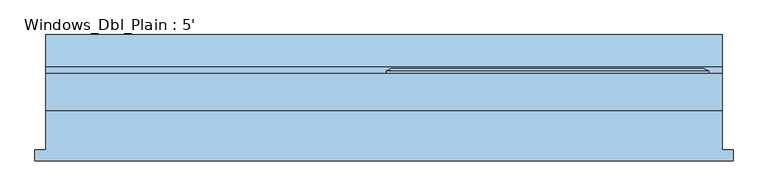
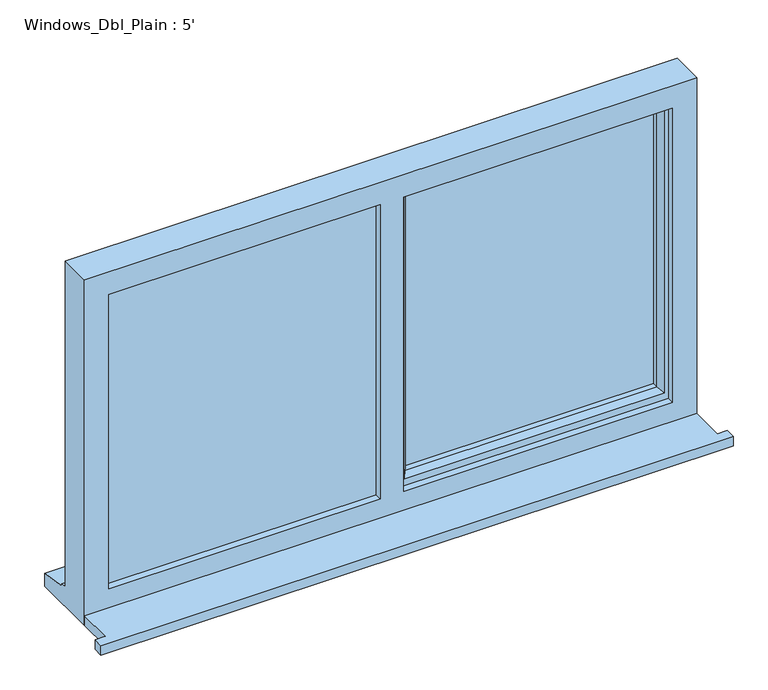
"""IFC4 building model written with IfcOpenShell, lengths in millimetres: window geometry, Windows_Dbl_Plain : 5'."""

from ifc_helpers import new_model, si_unit, frame, origin, place, context, project, spatial, polyline, outline, extrude, faceted_brep, source, transform, mapped, element, save


def windows_dbl_plain_5_93ba300c(model_context):
    return source(origin(), model_context, "Body", "SolidModel", [
        extrude(outline(polyline([(-1072.0, -127.7954322), (-1072.0, -102.7954322), (-1047.0, -102.7954322), (-1047.0, -13.2914322), (477.0, -13.2914322), (477.0, -102.7954322), (502.0, -102.7954322), (502.0, -127.7954322), (-1072.0, -127.7954322)])), frame((0.0, 0.0, 1200.0), z_axis=(0.0, 0.0, 1.0), x_axis=(1.0, 0.0, 0.0)), (0.0, 0.0, 1.0), 25.0),
        faceted_brep([(-280.0, 69.7085678, 2080.0), (-280.0, 75.4820705, 2080.0), (-280.0, 75.4820705, 1253.0), (-280.0, 69.7085678, 1253.0), (-270.0, 4.7085678, 2070.0), (-270.0, 69.7085678, 2070.0), (-270.0, 69.7085678, 1263.0), (-270.0, 4.7085678, 1263.0), (-230.0, 19.2014677, 2030.0), (-240.1480377, 4.7085678, 2040.1480377), (-240.1480377, 4.7085678, 1292.8519623), (-230.0, 19.2014677, 1303.0), (-230.0, 33.7085678, 2030.0), (-230.0, 33.7085678, 1303.0), (-240.0, 57.7085678, 2040.0), (-240.0, 33.7085678, 2040.0), (-240.0, 33.7085678, 1293.0), (-240.0, 57.7085678, 1293.0), (-230.0, 75.4820705, 2030.0), (-230.0, 57.7085678, 2030.0), (-230.0, 57.7085678, 1303.0), (-230.0, 75.4820705, 1303.0), (-247.4457548, 81.2555732, 2047.4457548), (-247.4457548, 81.2555732, 1285.5542452), (-269.2153903, 81.2555732, 2069.2153903), (-269.2153903, 81.2555732, 1263.7846097), (447.0, 75.4820705, 1253.0), (447.0, 69.7085678, 1253.0), (437.0, 69.7085678, 1263.0), (437.0, 4.7085678, 1263.0), (407.1480377, 4.7085678, 1292.8519623), (397.0, 19.2014677, 1303.0), (397.0, 33.7085678, 1303.0), (407.0, 33.7085678, 1293.0), (407.0, 57.7085678, 1293.0), (397.0, 57.7085678, 1303.0), (397.0, 75.4820705, 1303.0), (414.4457548, 81.2555732, 1285.5542452), (436.2153903, 81.2555732, 1263.7846097), (447.0, 75.4820705, 2080.0), (447.0, 69.7085678, 2080.0), (437.0, 69.7085678, 2070.0), (437.0, 4.7085678, 2070.0), (407.1480377, 4.7085678, 2040.1480377), (397.0, 19.2014677, 2030.0), (397.0, 33.7085678, 2030.0), (407.0, 33.7085678, 2040.0), (407.0, 57.7085678, 2040.0), (397.0, 57.7085678, 2030.0), (397.0, 75.4820705, 2030.0), (414.4457548, 81.2555732, 2047.4457548), (436.2153903, 81.2555732, 2069.2153903)], [[[0, 1, 2, 3]], [[4, 5, 6, 7]], [[8, 9, 10, 11]], [[12, 8, 11, 13]], [[14, 15, 16, 17]], [[18, 19, 20, 21]], [[22, 18, 21, 23]], [[1, 24, 25, 2]], [[3, 2, 26, 27]], [[7, 6, 28, 29]], [[11, 10, 30, 31]], [[13, 11, 31, 32]], [[17, 16, 33, 34]], [[21, 20, 35, 36]], [[23, 21, 36, 37]], [[2, 25, 38, 26]], [[27, 26, 39, 40]], [[29, 28, 41, 42]], [[31, 30, 43, 44]], [[32, 31, 44, 45]], [[34, 33, 46, 47]], [[36, 35, 48, 49]], [[37, 36, 49, 50]], [[26, 38, 51, 39]], [[40, 39, 1, 0]], [[3, 27, 40, 0], [5, 41, 28, 6]], [[42, 41, 5, 4]], [[7, 29, 42, 4], [9, 43, 30, 10]], [[44, 43, 9, 8]], [[45, 44, 8, 12]], [[15, 46, 33, 16], [13, 32, 45, 12]], [[47, 46, 15, 14]], [[17, 34, 47, 14], [19, 48, 35, 20]], [[49, 48, 19, 18]], [[50, 49, 18, 22]], [[24, 51, 38, 25], [23, 37, 50, 22]], [[39, 51, 24, 1]]]),
        extrude(outline(polyline([(2050.0, -310.0), (2070.0, -310.0), (2070.0, -1007.0), (1263.0, -1007.0), (1263.0, -310.0), (1283.0, -310.0), (1283.0, -987.0), (2050.0, -987.0), (2050.0, -310.0)])), frame((0.0, 28.7085678, 0.0), z_axis=(0.0, 1.0, 0.0), x_axis=(0.0, 0.0, 1.0)), (0.0, 0.0, 1.0), 41.0),
        faceted_brep([(477.0, -13.2914322, 2110.0), (-1047.0, -13.2914322, 2110.0), (-1047.0, -13.2914322, 1200.0), (477.0, -13.2914322, 1200.0), (417.0, -13.2914322, 2050.0), (417.0, -13.2914322, 1275.0), (-252.0, -13.2914322, 1275.0), (-252.0, -13.2914322, 2050.0), (-310.0, -13.2914322, 2050.0), (-310.0, -13.2914322, 1275.0), (-987.0, -13.2914322, 1275.0), (-987.0, -13.2914322, 2050.0), (-1047.0, 69.7085678, 2110.0), (-1047.0, 69.7085678, 1251.0), (-1047.0, 84.7085678, 1249.68767), (-1047.0, 84.7085678, 1244.7449676), (-1047.0, 157.2085678, 1233.8088847), (-1047.0, 157.2085678, 1200.0), (477.0, 69.7085678, 2110.0), (477.0, 69.7085678, 1251.0), (-1007.0, 69.7085678, 2070.0), (-1007.0, 69.7085678, 1263.0), (-310.0, 69.7085678, 1263.0), (-310.0, 69.7085678, 2070.0), (-270.0, 69.7085678, 2070.0), (-270.0, 69.7085678, 1263.0), (437.0, 69.7085678, 1263.0), (437.0, 69.7085678, 2070.0), (-1007.0, 4.7085678, 2070.0), (-1007.0, 4.7085678, 1263.0), (-300.0, 4.7085678, 2070.0), (-300.0, 4.7085678, 1263.0), (-310.0, 4.7085678, 2050.0), (-987.0, 4.7085678, 2050.0), (-987.0, 4.7085678, 1275.0), (-310.0, 4.7085678, 1275.0), (-270.0, 4.7085678, 2070.0), (437.0, 4.7085678, 2070.0), (437.0, 4.7085678, 1263.0), (-270.0, 4.7085678, 1263.0), (417.0, 4.7085678, 2050.0), (-252.0, 4.7085678, 2050.0), (-252.0, 4.7085678, 1275.0), (417.0, 4.7085678, 1275.0), (-310.0, 28.7085678, 2070.0), (-300.0, 28.7085678, 2070.0), (477.0, 157.2085678, 1200.0), (477.0, 157.2085678, 1233.8088847), (477.0, 84.7085678, 1244.7449676), (477.0, 84.7085678, 1249.68767), (-300.0, 28.7085678, 1263.0), (-310.0, 28.7085678, 1263.0)], [[[0, 1, 2, 3], [4, 5, 6, 7], [8, 9, 10, 11]], [[2, 1, 12, 13, 14, 15, 16, 17]], [[13, 12, 18, 19], [20, 21, 22, 23], [24, 25, 26, 27]], [[21, 20, 28, 29]], [[28, 30, 31, 29], [32, 33, 34, 35]], [[36, 37, 38, 39], [40, 41, 42, 43]], [[33, 11, 10, 34]], [[1, 0, 18, 12]], [[28, 20, 23, 44, 45, 30]], [[27, 37, 36, 24]], [[11, 33, 32, 8]], [[40, 4, 7, 41]], [[19, 18, 0, 3, 46, 47, 48, 49]], [[27, 26, 38, 37]], [[4, 40, 43, 5]], [[45, 50, 31, 30]], [[50, 45, 44, 51]], [[51, 44, 23, 22]], [[25, 24, 36, 39]], [[41, 7, 6, 42]], [[8, 32, 35, 9]], [[46, 3, 2, 17]], [[47, 46, 17, 16]], [[48, 47, 16, 15]], [[49, 48, 15, 14]], [[19, 49, 14, 13]], [[22, 21, 29, 31, 50, 51]], [[26, 25, 39, 38]], [[6, 5, 43, 42]], [[35, 34, 10, 9]]]),
        extrude(outline(polyline([(-1007.0, 28.7085678), (-300.0, 28.7085678), (-300.0, 4.7085678), (-1007.0, 4.7085678), (-1007.0, 28.7085678)])), frame((0.0, 0.0, 1263.0), z_axis=(0.0, 0.0, 1.0), x_axis=(1.0, 0.0, 0.0)), (0.0, 0.0, 1.0), 807.0),
        extrude(outline(polyline([(407.0, 33.7085678), (-240.0, 33.7085678), (-240.0, 57.7085678), (407.0, 57.7085678), (407.0, 33.7085678)])), frame((0.0, 0.0, 1293.0), z_axis=(0.0, 0.0, 1.0), x_axis=(1.0, 0.0, 0.0)), (0.0, 0.0, 1.0), 747.0),
    ])


if __name__ == "__main__":
    model = new_model("IFC4")
    model_context = context("Model", 3, world=origin())
    ifc_project = project(units=[si_unit("LENGTHUNIT", "METRE", prefix="MILLI")], contexts=[model_context])
    site = spatial("IfcSite", under=ifc_project)
    building = spatial("IfcBuilding", under=site)
    placement = place(None, origin())
    windows_dbl_plain_5_shape = windows_dbl_plain_5_93ba300c(model_context)
    element("IfcWindow", 1, ObjectType="Windows_Dbl_Plain : 5'", at=placement, inside=building, context=model_context, shape_type="MappedRepresentation", body=[
        mapped(windows_dbl_plain_5_shape, transform((0.0, 0.0, 0.0), x_axis=(1.0, 0.0, 0.0), y_axis=(0.0, 1.0, 0.0), z_axis=(0.0, 0.0, 1.0))),
    ])
    save(model, "model.ifc")

# Revit data of these elements
# Type "Windows_Dbl_Plain : 5'"
#   Type Mark = "58"
#   Operation = "DoublePanelVertical"
#   Construction Type Id = "GSP4R"
#   Manufacturer = "Revit"
#   Keynote = "L10"
#   Analytic Construction = "1/8 in Pilkington single glazing"
#   Wrap Layers (Ext) from Ext = 0.336286 ft
#   Wrap Layers (Int) from Ext = 0.582349 ft
#   Window Board Projection = 0.082021 ft
#   Window Board Extension = 0.082021 ft
#   Visual Light Transmittance = 0.9
#   Solar Heat Gain Coefficient = 0.78
#   Rough Width = 5.0 ft
#   Rough Height = 2.985564 ft
#   Height = 2.985564 ft
#   Width = 5.0 ft
#   Heat Transfer Coefficient (U) = 3.6886 W/(m²·K)
#   Glazing Thickness = 0.07874 ft
#   FrameOffset - External = 0.164042 ft
#   Frame Depth = 0.213255 ft
#   Default Head Height = 6.922572 ft
#   Cill Depth = 0.287073 ft
#   Cavity Closer Width = 0.164042 ft
#   Cavity Closer Offset from Ext = 0.336286 ft
#   Cavity Closer Depth = 0.278871 ft
#   Vis - Cavity Closers = yes
#   Define Thermal Properties by = 1
#   Material Trim = Window Frame
#   Material Glass = Glass
#   Material Frame = Window Frame
#   Wall Closure = (empty or 0)
# Element 1 (IfcWindow, "Windows_Dbl_Plain : 5'")
#   Materials on its faces: "Window Frame", "Glass"
# Materials
#   "Window Frame": colour RGB 249 249 249, transparency 0, Keynote = "L10", Cost = 0
#   "Glass": class "Glass", colour RGB 0 128 192, transparency 0.9, Description = "Soda Lime Glass", Cost = 0
